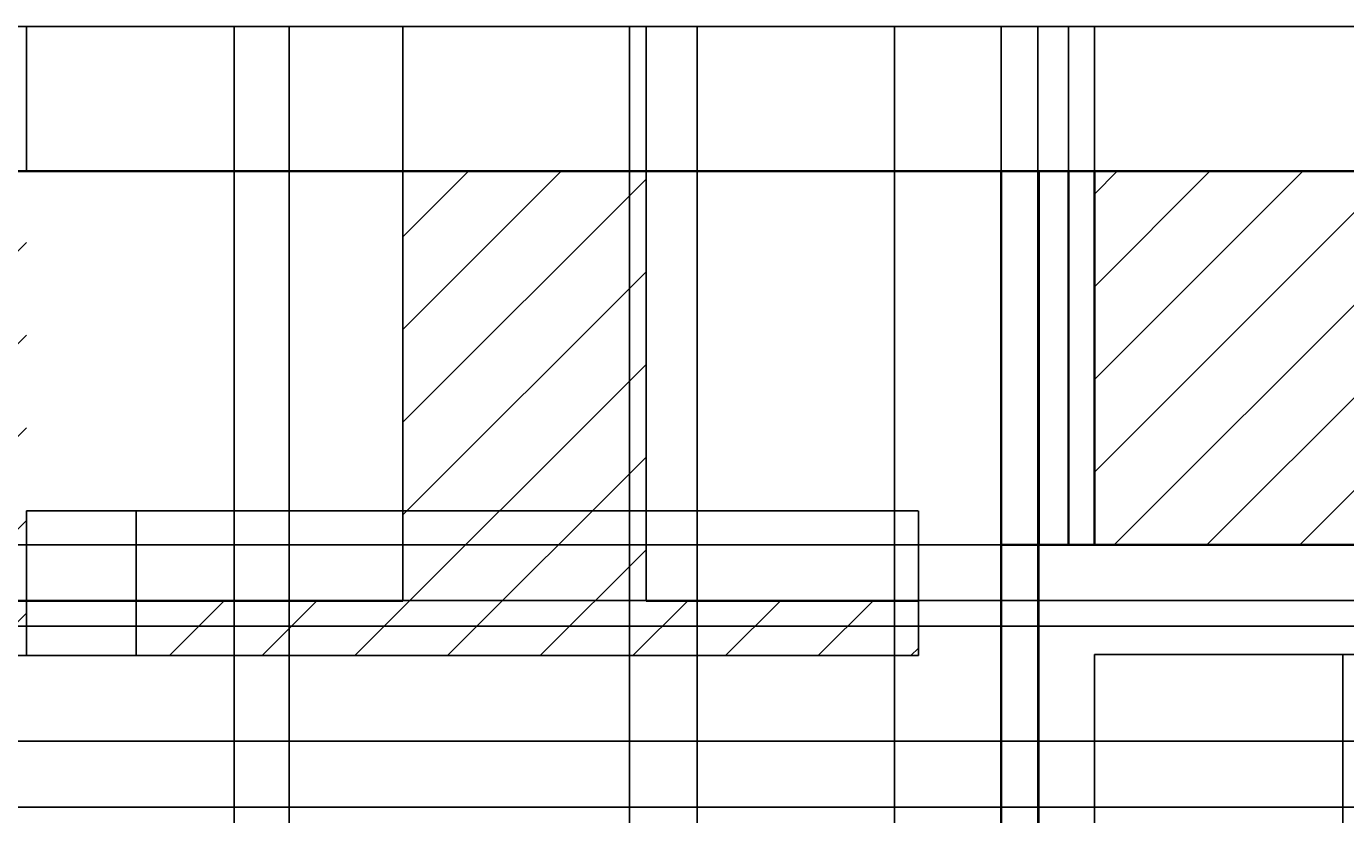
# Model space of a CAD drawing. Units: millimetres. Extents: x 2212 to 7718, y 1114 to 4219.
# Tile 4 of 5: x 4165 to 6466, y 2844 to 4219. Entities that reach past the tile are written whole.
import ezdxf

# ---------------------------------------------------------------- set-up
doc = ezdxf.new("R2010")
doc.units = ezdxf.units.MM
for name, color, linetype, lineweight in [('A-ANNO-DIMS', 2, 'Continuous', 18), ('A-ELEV-PATT', 8, 'Continuous', 13), ('A-EQPM', 4, 'Continuous', 25), ('A-FURN', 7, 'Continuous', 35)]:
    doc.layers.add(name, color=color, linetype=linetype, lineweight=lineweight)
doc.styles.get("Standard").update_dxf_attribs({"font": 'arial.ttf'})
doc.dimstyles.get("Standard").update_dxf_attribs({"dimtxt": 0.18, "dimasz": 0.18, "dimexe": 0.18, "dimexo": 0.0625, "dimgap": 0.09, "dimtad": 0, "dimtih": 1, "dimtoh": 1, "dimdec": 4, "dimzin": 0, "dimdsep": 46, "dimtxsty": 'Standard', "dimcen": 0.09, "dimadec": 0, "dimazin": 0, "dimtfac": 1, "dimtdec": 4, "dimtofl": 0, "dimtmove": 0, "dimatfit": 3, "dimfxl": 1, "dimtolj": 1, "dimtzin": 0, "dimarcsym": 0})

# ---------------------------------------------------------------- blocks, each defined once
blk = doc.blocks.new('*D3')
at = {"layer": 'A-ANNO-DIMS', "color": 0, "lineweight": -2, "transparency": 16777216}
for p, q in [((3659.3, 3966.2), (3659.3, 4218.9)), ((3659.5, 4218.7), (3911.8, 4218.7)), ((4165, 4218.7), (3912.6, 4218.7)), ((4165.1, 3966.2), (4165.1, 4218.9))]:
    blk.add_line(p, q, dxfattribs=at)
at = {"layer": 'A-ANNO-DIMS', "color": 0, "transparency": 16777216}
for points in [[(3659.5, 4218.7), (3659.5, 4218.7), (3659.3, 4218.7)], [(4165, 4218.7), (4165, 4218.7), (4165.1, 4218.7)]]:
    blk.add_solid(points, dxfattribs=at)
at = {"layer": 'Defpoints', "color": 0, "transparency": 16777216}
for p in [(4165.1, 4218.7), (3659.3, 3966.2), (4165.1, 3966.2)]:
    blk.add_point(p, dxfattribs=at)
at = {"layer": 'A-ANNO-DIMS', "color": 0, "transparency": 16777216, "insert": (3912.2, 4218.7), "char_height": 0.18, "attachment_point": 5}
blk.add_mtext('\\A1;505.8', dxfattribs=at)
blk = doc.blocks.new('*D4')
at = {"layer": 'A-ANNO-DIMS', "color": 0, "lineweight": -2, "transparency": 16777216}
for p, q in [((4165.1, 3966.2), (4165.1, 4218.9)), ((4165.3, 4218.7), (4493, 4218.7)), ((4821.4, 4218.7), (4493.8, 4218.7)), ((4821.6, 3966.2), (4821.6, 4218.9))]:
    blk.add_line(p, q, dxfattribs=at)
at = {"layer": 'A-ANNO-DIMS', "color": 0, "transparency": 16777216}
for points in [[(4165.3, 4218.7), (4165.3, 4218.7), (4165.1, 4218.7)], [(4821.4, 4218.7), (4821.4, 4218.7), (4821.6, 4218.7)]]:
    blk.add_solid(points, dxfattribs=at)
at = {"layer": 'Defpoints', "color": 0, "transparency": 16777216}
for p in [(4821.6, 4218.7), (4165.1, 3966.2), (4821.6, 3966.2)]:
    blk.add_point(p, dxfattribs=at)
at = {"layer": 'A-ANNO-DIMS', "color": 0, "transparency": 16777216, "insert": (4493.4, 4218.7), "char_height": 0.18, "attachment_point": 5}
blk.add_mtext('\\A1;656.4', dxfattribs=at)
blk = doc.blocks.new('*D5')
at = {"layer": 'A-ANNO-DIMS', "color": 0, "lineweight": -2, "transparency": 16777216}
for p, q in [((4821.6, 3966.2), (4821.6, 4218.9)), ((4821.8, 4218.7), (5033.2, 4218.7)), ((5245.6, 4218.7), (5034.1, 4218.7)), ((5245.7, 3966.2), (5245.7, 4218.9))]:
    blk.add_line(p, q, dxfattribs=at)
at = {"layer": 'A-ANNO-DIMS', "color": 0, "transparency": 16777216}
for points in [[(4821.8, 4218.7), (4821.8, 4218.7), (4821.6, 4218.7)], [(5245.6, 4218.7), (5245.6, 4218.7), (5245.7, 4218.7)]]:
    blk.add_solid(points, dxfattribs=at)
at = {"layer": 'Defpoints', "color": 0, "transparency": 16777216}
for p in [(5245.7, 4218.7), (4821.6, 3966.2), (5245.7, 3966.2)]:
    blk.add_point(p, dxfattribs=at)
at = {"layer": 'A-ANNO-DIMS', "color": 0, "transparency": 16777216, "insert": (5033.7, 4218.7), "char_height": 0.18, "attachment_point": 5}
blk.add_mtext('\\A1;424.15', dxfattribs=at)
blk = doc.blocks.new('*D6')
at = {"layer": 'A-ANNO-DIMS', "color": 0, "lineweight": -2, "transparency": 16777216}
for p, q in [((5245.7, 3966.2), (5245.7, 4218.9)), ((5245.9, 4218.7), (5555, 4218.7)), ((5865, 4218.7), (5555.8, 4218.7)), ((5865.1, 3966.2), (5865.1, 4218.9))]:
    blk.add_line(p, q, dxfattribs=at)
at = {"layer": 'A-ANNO-DIMS', "color": 0, "transparency": 16777216}
for points in [[(5245.9, 4218.7), (5245.9, 4218.7), (5245.7, 4218.7)], [(5865, 4218.7), (5865, 4218.7), (5865.1, 4218.7)]]:
    blk.add_solid(points, dxfattribs=at)
at = {"layer": 'Defpoints', "color": 0, "transparency": 16777216}
for p in [(5865.1, 4218.7), (5245.7, 3966.2), (5865.1, 3966.2)]:
    blk.add_point(p, dxfattribs=at)
at = {"layer": 'A-ANNO-DIMS', "color": 0, "transparency": 16777216, "insert": (5555.4, 4218.7), "char_height": 0.18, "attachment_point": 5}
blk.add_mtext('\\A1;619.4', dxfattribs=at)
blk = doc.blocks.new('*D7')
at = {"layer": 'A-ANNO-DIMS', "color": 0, "lineweight": -2, "transparency": 16777216}
for p, q in [((5865.1, 3966.2), (5865.1, 4218.9)), ((5865.3, 4218.7), (6264.9, 4218.7)), ((6665, 4218.7), (6265.4, 4218.7)), ((6665.1, 3966.2), (6665.1, 4218.9))]:
    blk.add_line(p, q, dxfattribs=at)
at = {"layer": 'A-ANNO-DIMS', "color": 0, "transparency": 16777216}
for points in [[(5865.3, 4218.7), (5865.3, 4218.7), (5865.1, 4218.7)], [(6665, 4218.7), (6665, 4218.7), (6665.1, 4218.7)]]:
    blk.add_solid(points, dxfattribs=at)
at = {"layer": 'Defpoints', "color": 0, "transparency": 16777216}
for p in [(6665.1, 4218.7), (5865.1, 3966.2), (6665.1, 3966.2)]:
    blk.add_point(p, dxfattribs=at)
at = {"layer": 'A-ANNO-DIMS', "color": 0, "transparency": 16777216, "insert": (6265.1, 4218.7), "char_height": 0.18, "attachment_point": 5}
blk.add_mtext('\\A1;800', dxfattribs=at)
blk = doc.blocks.new('*D10')
at = {"layer": 'A-ANNO-DIMS', "color": 0, "lineweight": -2, "transparency": 16777216}
for p, q in [((4165.1, 3121.4), (4165.1, 3374)), ((4165.3, 3373.8), (4260.5, 3373.8)), ((4356.5, 3373.8), (4261.4, 3373.8)), ((4356.7, 3121.4), (4356.7, 3374))]:
    blk.add_line(p, q, dxfattribs=at)
at = {"layer": 'A-ANNO-DIMS', "color": 0, "transparency": 16777216}
for points in [[(4165.3, 3373.9), (4165.3, 3373.8), (4165.1, 3373.8)], [(4356.5, 3373.9), (4356.5, 3373.8), (4356.7, 3373.8)]]:
    blk.add_solid(points, dxfattribs=at)
at = {"layer": 'Defpoints', "color": 0, "transparency": 16777216}
for p in [(4356.7, 3373.8), (4165.1, 3121.3), (4356.7, 3121.3)]:
    blk.add_point(p, dxfattribs=at)
at = {"layer": 'A-ANNO-DIMS', "color": 0, "transparency": 16777216, "insert": (4260.9, 3373.8), "char_height": 0.18, "attachment_point": 5}
blk.add_mtext('\\A1;191.58', dxfattribs=at)
blk = doc.blocks.new('*D11')
at = {"layer": 'A-ANNO-DIMS', "color": 0, "lineweight": -2, "transparency": 16777216}
for p, q in [((4356.7, 3121.4), (4356.7, 3374)), ((4356.9, 3373.8), (5038.4, 3373.8)), ((5720.6, 3373.8), (5039.1, 3373.8)), ((5720.8, 3121.4), (5720.8, 3374))]:
    blk.add_line(p, q, dxfattribs=at)
at = {"layer": 'A-ANNO-DIMS', "color": 0, "transparency": 16777216}
for points in [[(4356.9, 3373.9), (4356.9, 3373.8), (4356.7, 3373.8)], [(5720.6, 3373.9), (5720.6, 3373.8), (5720.8, 3373.8)]]:
    blk.add_solid(points, dxfattribs=at)
at = {"layer": 'Defpoints', "color": 0, "transparency": 16777216}
for p in [(5720.8, 3373.8), (4356.7, 3121.3), (5720.8, 3121.3)]:
    blk.add_point(p, dxfattribs=at)
at = {"layer": 'A-ANNO-DIMS', "color": 0, "transparency": 16777216, "insert": (5038.7, 3373.8), "char_height": 0.18, "attachment_point": 5}
blk.add_mtext('\\A1;1364', dxfattribs=at)
blk = doc.blocks.new('*D12')
at = {"layer": 'A-ANNO-DIMS', "color": 0, "lineweight": -2, "transparency": 16777216}
for p, q in [((4356.7, 3216.4), (4104, 3216.4)), ((4104.2, 3216.2), (4104.2, 3169)), ((4104.2, 3121.5), (4104.2, 3168.7)), ((4356.7, 3121.3), (4104, 3121.3))]:
    blk.add_line(p, q, dxfattribs=at)
at = {"layer": 'A-ANNO-DIMS', "color": 0, "transparency": 16777216}
for points in [[(4104.2, 3216.2), (4104.2, 3216.2), (4104.2, 3216.4)], [(4104.2, 3121.5), (4104.2, 3121.5), (4104.2, 3121.3)]]:
    blk.add_solid(points, dxfattribs=at)
at = {"layer": 'Defpoints', "color": 0, "transparency": 16777216}
for p in [(4104.2, 3216.4), (4356.7, 3216.4), (4356.7, 3121.3)]:
    blk.add_point(p, dxfattribs=at)
at = {"layer": 'A-ANNO-DIMS', "color": 0, "transparency": 16777216, "insert": (4104.2, 3168.9), "char_height": 0.18, "attachment_point": 5}
blk.add_mtext('\\A1;95.06', dxfattribs=at)
blk = doc.blocks.new('*D28')
at = {"layer": 'A-ANNO-DIMS', "color": 0, "lineweight": -2, "transparency": 16777216}
for p, q in [((5865.1, 2856.7), (2212.5, 2856.7)), ((2212.6, 2856.6), (2212.6, 2802)), ((2212.6, 2747), (2212.6, 2801.6)), ((5865.1, 2746.8), (2212.5, 2746.8))]:
    blk.add_line(p, q, dxfattribs=at)
at = {"layer": 'A-ANNO-DIMS', "color": 0, "transparency": 16777216}
for points in [[(2212.6, 2856.6), (2212.7, 2856.6), (2212.6, 2856.7)], [(2212.6, 2747), (2212.7, 2747), (2212.6, 2746.8)]]:
    blk.add_solid(points, dxfattribs=at)
at = {"layer": 'Defpoints', "color": 0, "transparency": 16777216}
for p in [(2212.6, 2856.7), (5865.1, 2856.7), (5865.1, 2746.8)]:
    blk.add_point(p, dxfattribs=at)
at = {"layer": 'A-ANNO-DIMS', "color": 0, "transparency": 16777216, "insert": (2212.6, 2801.8), "char_height": 0.18, "attachment_point": 5}
blk.add_mtext('\\A1;109.95', dxfattribs=at)
blk = doc.blocks.new('*D29')
at = {"layer": 'A-ANNO-DIMS', "color": 0, "lineweight": -2, "transparency": 16777216}
for p, q in [((5865.1, 3217.2), (2212.5, 3217.2)), ((2212.6, 3217.1), (2212.6, 3037.2)), ((2212.6, 2856.9), (2212.6, 3036.8)), ((5865.1, 2856.7), (2212.5, 2856.7))]:
    blk.add_line(p, q, dxfattribs=at)
at = {"layer": 'A-ANNO-DIMS', "color": 0, "transparency": 16777216}
for points in [[(2212.6, 3217.1), (2212.7, 3217.1), (2212.6, 3217.2)], [(2212.6, 2856.9), (2212.7, 2856.9), (2212.6, 2856.7)]]:
    blk.add_solid(points, dxfattribs=at)
at = {"layer": 'Defpoints', "color": 0, "transparency": 16777216}
for p in [(2212.6, 3217.2), (5865.1, 3217.2), (5865.1, 2856.7)]:
    blk.add_point(p, dxfattribs=at)
at = {"layer": 'A-ANNO-DIMS', "color": 0, "transparency": 16777216, "insert": (2212.6, 3037), "char_height": 0.18, "attachment_point": 5}
blk.add_mtext('\\A1;360.5', dxfattribs=at)
blk = doc.blocks.new('*D30')
at = {"layer": 'A-ANNO-DIMS', "color": 0, "lineweight": -2, "transparency": 16777216}
for p, q in [((5865.1, 3314.4), (2212.5, 3314.4)), ((2212.6, 3314.2), (2212.6, 3266)), ((2212.6, 3217.4), (2212.6, 3265.6)), ((5865.1, 3217.2), (2212.5, 3217.2))]:
    blk.add_line(p, q, dxfattribs=at)
at = {"layer": 'A-ANNO-DIMS', "color": 0, "transparency": 16777216}
for points in [[(2212.6, 3314.2), (2212.7, 3314.2), (2212.6, 3314.4)], [(2212.6, 3217.4), (2212.7, 3217.4), (2212.6, 3217.2)]]:
    blk.add_solid(points, dxfattribs=at)
at = {"layer": 'Defpoints', "color": 0, "transparency": 16777216}
for p in [(2212.6, 3314.4), (5865.1, 3314.4), (5865.1, 3217.2)]:
    blk.add_point(p, dxfattribs=at)
at = {"layer": 'A-ANNO-DIMS', "color": 0, "transparency": 16777216, "insert": (2212.6, 3265.8), "char_height": 0.18, "attachment_point": 5}
blk.add_mtext('\\A1;97.14', dxfattribs=at)
blk = doc.blocks.new('*D31')
at = {"layer": 'A-ANNO-DIMS', "color": 0, "lineweight": -2, "transparency": 16777216}
for p, q in [((5865.1, 3966.2), (2212.5, 3966.2)), ((2212.6, 3966), (2212.6, 3640.5)), ((2212.6, 3314.6), (2212.6, 3640.1)), ((5865.1, 3314.4), (2212.5, 3314.4))]:
    blk.add_line(p, q, dxfattribs=at)
at = {"layer": 'A-ANNO-DIMS', "color": 0, "transparency": 16777216}
for points in [[(2212.6, 3966), (2212.7, 3966), (2212.6, 3966.2)], [(2212.6, 3314.6), (2212.7, 3314.6), (2212.6, 3314.4)]]:
    blk.add_solid(points, dxfattribs=at)
at = {"layer": 'Defpoints', "color": 0, "transparency": 16777216}
for p in [(2212.6, 3966.2), (5865.1, 3966.2), (5865.1, 3314.4)]:
    blk.add_point(p, dxfattribs=at)
at = {"layer": 'A-ANNO-DIMS', "color": 0, "transparency": 16777216, "insert": (2212.6, 3640.3), "char_height": 0.18, "attachment_point": 5}
blk.add_mtext('\\A1;651.8', dxfattribs=at)
blk = doc.blocks.new('*D32')
at = {"layer": 'A-ANNO-DIMS', "color": 0, "lineweight": -2, "transparency": 16777216}
for p, q in [((5865.1, 3314.3), (5865.1, 1113.5)), ((5930.5, 3314.3), (5930.5, 1113.5)), ((5865.3, 1113.7), (5897.4, 1113.7)), ((5930.3, 1113.7), (5898.2, 1113.7))]:
    blk.add_line(p, q, dxfattribs=at)
at = {"layer": 'A-ANNO-DIMS', "color": 0, "transparency": 16777216}
for points in [[(5865.3, 1113.7), (5865.3, 1113.7), (5865.1, 1113.7)], [(5930.3, 1113.7), (5930.3, 1113.7), (5930.5, 1113.7)]]:
    blk.add_solid(points, dxfattribs=at)
at = {"layer": 'Defpoints', "color": 0, "transparency": 16777216}
for p in [(5865.1, 3314.4), (5930.5, 3314.4), (5930.5, 1113.7)]:
    blk.add_point(p, dxfattribs=at)
at = {"layer": 'A-ANNO-DIMS', "color": 0, "transparency": 16777216, "insert": (5897.8, 1113.7), "char_height": 0.18, "attachment_point": 5}
blk.add_mtext('\\A1;65.32', dxfattribs=at)
blk = doc.blocks.new('*D33')
at = {"layer": 'A-ANNO-DIMS', "color": 0, "lineweight": -2, "transparency": 16777216}
for p, q in [((5865.1, 3314.4), (5865.1, 4218.9)), ((5865.3, 4218.7), (5923.5, 4218.7)), ((5982.4, 4218.7), (5924.2, 4218.7)), ((5982.5, 3314.4), (5982.5, 4218.9))]:
    blk.add_line(p, q, dxfattribs=at)
at = {"layer": 'A-ANNO-DIMS', "color": 0, "transparency": 16777216}
for points in [[(5865.3, 4218.7), (5865.3, 4218.7), (5865.1, 4218.7)], [(5982.4, 4218.7), (5982.4, 4218.7), (5982.5, 4218.7)]]:
    blk.add_solid(points, dxfattribs=at)
at = {"layer": 'Defpoints', "color": 0, "transparency": 16777216}
for p in [(5982.5, 4218.7), (5865.1, 3314.4), (5982.5, 3314.4)]:
    blk.add_point(p, dxfattribs=at)
at = {"layer": 'A-ANNO-DIMS', "color": 0, "transparency": 16777216, "insert": (5923.8, 4218.7), "char_height": 0.18, "attachment_point": 5}
blk.add_mtext('\\A1;117.4', dxfattribs=at)
blk = doc.blocks.new('*D34')
at = {"layer": 'A-ANNO-DIMS', "color": 0, "lineweight": -2, "transparency": 16777216}
for p, q in [((5982.5, 3314.4), (5982.5, 4218.9)), ((5982.7, 4218.7), (6004.8, 4218.7)), ((6027.6, 4218.7), (6005.6, 4218.7)), ((6027.8, 3314.4), (6027.8, 4218.9))]:
    blk.add_line(p, q, dxfattribs=at)
at = {"layer": 'A-ANNO-DIMS', "color": 0, "transparency": 16777216}
for points in [[(5982.7, 4218.7), (5982.7, 4218.7), (5982.5, 4218.7)], [(6027.6, 4218.7), (6027.6, 4218.7), (6027.8, 4218.7)]]:
    blk.add_solid(points, dxfattribs=at)
at = {"layer": 'Defpoints', "color": 0, "transparency": 16777216}
for p in [(6027.8, 4218.7), (5982.5, 3314.4), (6027.8, 3314.4)]:
    blk.add_point(p, dxfattribs=at)
at = {"layer": 'A-ANNO-DIMS', "color": 0, "transparency": 16777216, "insert": (6005.2, 4218.7), "char_height": 0.18, "attachment_point": 5}
blk.add_mtext('\\A1;45.24', dxfattribs=at)
blk = doc.blocks.new('*D35')
at = {"layer": 'A-ANNO-DIMS', "color": 0, "lineweight": -2, "transparency": 16777216}
for p, q in [((6027.8, 2972.1), (6027.8, 1113.5)), ((6460.8, 2972.1), (6460.8, 1113.5)), ((6028, 1113.7), (6244, 1113.7)), ((6460.6, 1113.7), (6244.6, 1113.7))]:
    blk.add_line(p, q, dxfattribs=at)
at = {"layer": 'A-ANNO-DIMS', "color": 0, "transparency": 16777216}
for points in [[(6028, 1113.7), (6028, 1113.7), (6027.8, 1113.7)], [(6460.6, 1113.7), (6460.6, 1113.7), (6460.8, 1113.7)]]:
    blk.add_solid(points, dxfattribs=at)
at = {"layer": 'Defpoints', "color": 0, "transparency": 16777216}
for p in [(6027.8, 2972.2), (6460.8, 2972.2), (6460.8, 1113.7)]:
    blk.add_point(p, dxfattribs=at)
at = {"layer": 'A-ANNO-DIMS', "color": 0, "transparency": 16777216, "insert": (6244.3, 1113.7), "char_height": 0.18, "attachment_point": 5}
blk.add_mtext('\\A1;433', dxfattribs=at)
blk = doc.blocks.new('*D36')
at = {"layer": 'A-ANNO-DIMS', "color": 0, "lineweight": -2, "transparency": 16777216}
for p, q in [((6460.9, 3122.9), (7717.8, 3122.9)), ((7717.6, 3122.7), (7717.6, 3047.7)), ((7717.6, 2972.4), (7717.6, 3047.3)), ((6460.9, 2972.2), (7717.8, 2972.2))]:
    blk.add_line(p, q, dxfattribs=at)
at = {"layer": 'A-ANNO-DIMS', "color": 0, "transparency": 16777216}
for points in [[(7717.6, 3122.7), (7717.7, 3122.7), (7717.6, 3122.9)], [(7717.6, 2972.4), (7717.7, 2972.4), (7717.6, 2972.2)]]:
    blk.add_solid(points, dxfattribs=at)
at = {"layer": 'Defpoints', "color": 0, "transparency": 16777216}
for p in [(6460.8, 3122.9), (7717.6, 3122.9), (6460.8, 2972.2)]:
    blk.add_point(p, dxfattribs=at)
at = {"layer": 'A-ANNO-DIMS', "color": 0, "transparency": 16777216, "insert": (7717.6, 3047.5), "char_height": 0.18, "attachment_point": 5}
blk.add_mtext('\\A1;150.68', dxfattribs=at)
blk = doc.blocks.new('*D37')
at = {"layer": 'A-ANNO-DIMS', "color": 0, "lineweight": -2, "transparency": 16777216}
for p, q in [((6027.7, 2972.2), (2212.5, 2972.2)), ((2212.6, 2972), (2212.6, 2914.6)), ((2212.6, 2856.9), (2212.6, 2914.3)), ((5930.4, 2856.7), (2212.5, 2856.7))]:
    blk.add_line(p, q, dxfattribs=at)
at = {"layer": 'A-ANNO-DIMS', "color": 0, "transparency": 16777216}
for points in [[(2212.6, 2972), (2212.7, 2972), (2212.6, 2972.2)], [(2212.6, 2856.9), (2212.7, 2856.9), (2212.6, 2856.7)]]:
    blk.add_solid(points, dxfattribs=at)
at = {"layer": 'Defpoints', "color": 0, "transparency": 16777216}
for p in [(2212.6, 2972.2), (6027.8, 2972.2), (5930.5, 2856.7)]:
    blk.add_point(p, dxfattribs=at)
at = {"layer": 'A-ANNO-DIMS', "color": 0, "transparency": 16777216, "insert": (2212.6, 2914.5), "char_height": 0.18, "attachment_point": 5}
blk.add_mtext('\\A1;115.44', dxfattribs=at)
blk = doc.blocks.new('*D42')
at = {"layer": 'A-ANNO-DIMS', "color": 0, "lineweight": -2, "transparency": 16777216}
for p, q in [((6506, 3217.2), (2212.5, 3217.2)), ((2212.6, 3217.1), (2212.6, 3195)), ((2212.6, 3172.6), (2212.6, 3194.6)), ((6530.4, 3172.4), (2212.5, 3172.4))]:
    blk.add_line(p, q, dxfattribs=at)
at = {"layer": 'A-ANNO-DIMS', "color": 0, "transparency": 16777216}
for points in [[(2212.6, 3217.1), (2212.7, 3217.1), (2212.6, 3217.2)], [(2212.6, 3172.6), (2212.7, 3172.6), (2212.6, 3172.4)]]:
    blk.add_solid(points, dxfattribs=at)
at = {"layer": 'Defpoints', "color": 0, "transparency": 16777216}
for p in [(6506.1, 3217.2), (2212.6, 3172.4), (6530.5, 3172.4)]:
    blk.add_point(p, dxfattribs=at)
at = {"layer": 'A-ANNO-DIMS', "color": 0, "transparency": 16777216, "insert": (2212.6, 3194.8), "char_height": 0.18, "attachment_point": 5}
blk.add_mtext('\\A1;44.855', dxfattribs=at)
blk = doc.blocks.new('*D50')
at = {"layer": 'A-ANNO-DIMS', "color": 0, "lineweight": -2, "transparency": 16777216}
for p, q in [((5865.1, 2746.9), (5865.1, 4218.9)), ((5865.3, 4218.7), (5896.7, 4218.7)), ((5928.9, 4218.7), (5897.5, 4218.7)), ((5929, 2684.6), (5929, 4218.9))]:
    blk.add_line(p, q, dxfattribs=at)
at = {"layer": 'A-ANNO-DIMS', "color": 0, "transparency": 16777216}
for points in [[(5865.3, 4218.7), (5865.3, 4218.7), (5865.1, 4218.7)], [(5928.9, 4218.7), (5928.9, 4218.7), (5929, 4218.7)]]:
    blk.add_solid(points, dxfattribs=at)
at = {"layer": 'Defpoints', "color": 0, "transparency": 16777216}
for p in [(5929, 4218.7), (5865.1, 2746.8), (5929, 2684.5)]:
    blk.add_point(p, dxfattribs=at)
at = {"layer": 'A-ANNO-DIMS', "color": 0, "transparency": 16777216, "insert": (5897.1, 4218.7), "char_height": 0.18, "attachment_point": 5}
blk.add_mtext('\\A1;63.91', dxfattribs=at)
blk = doc.blocks.new('*D69')
at = {"layer": 'A-ANNO-DIMS', "color": 0, "lineweight": -2, "transparency": 16777216}
for p, q in [((4623.4, 2414.9), (4623.4, 4218.9)), ((4623.6, 4218.7), (5150.6, 4218.7)), ((5678.7, 4218.7), (5151.6, 4218.7)), ((5678.9, 2414.9), (5678.9, 4218.9))]:
    blk.add_line(p, q, dxfattribs=at)
at = {"layer": 'A-ANNO-DIMS', "color": 0, "transparency": 16777216}
for points in [[(4623.6, 4218.7), (4623.6, 4218.7), (4623.4, 4218.7)], [(5678.7, 4218.7), (5678.7, 4218.7), (5678.9, 4218.7)]]:
    blk.add_solid(points, dxfattribs=at)
at = {"layer": 'Defpoints', "color": 0, "transparency": 16777216}
for p in [(5678.9, 4218.7), (4623.4, 2414.8), (5678.9, 2414.8)]:
    blk.add_point(p, dxfattribs=at)
at = {"layer": 'A-ANNO-DIMS', "color": 0, "transparency": 16777216, "insert": (5151.1, 4218.7), "char_height": 0.18, "attachment_point": 5}
blk.add_mtext('\\A1;1055.48', dxfattribs=at)
blk = doc.blocks.new('*D70')
at = {"layer": 'A-ANNO-DIMS', "color": 0, "lineweight": -2, "transparency": 16777216}
for p, q in [((4527.5, 2333.4), (4527.5, 4218.9)), ((4527.7, 4218.7), (4575.1, 4218.7)), ((4623.2, 4218.7), (4575.8, 4218.7)), ((4623.4, 2414.9), (4623.4, 4218.9))]:
    blk.add_line(p, q, dxfattribs=at)
at = {"layer": 'A-ANNO-DIMS', "color": 0, "transparency": 16777216}
for points in [[(4527.7, 4218.7), (4527.7, 4218.7), (4527.5, 4218.7)], [(4623.2, 4218.7), (4623.2, 4218.7), (4623.4, 4218.7)]]:
    blk.add_solid(points, dxfattribs=at)
at = {"layer": 'Defpoints', "color": 0, "transparency": 16777216}
for p in [(4623.4, 4218.7), (4623.4, 2414.8), (4527.5, 2333.4)]:
    blk.add_point(p, dxfattribs=at)
at = {"layer": 'A-ANNO-DIMS', "color": 0, "transparency": 16777216, "insert": (4575.4, 4218.7), "char_height": 0.18, "attachment_point": 5}
blk.add_mtext('\\A1;95.87', dxfattribs=at)
blk = doc.blocks.new('*D72')
at = {"layer": 'A-ANNO-DIMS', "color": 0, "lineweight": -2, "transparency": 16777216}
for p, q in [((5216.8, 2499.3), (5216.8, 4218.9)), ((5217, 4218.7), (5275.6, 4218.7)), ((5335, 4218.7), (5276.5, 4218.7)), ((5335.2, 2499.3), (5335.2, 4218.9))]:
    blk.add_line(p, q, dxfattribs=at)
at = {"layer": 'A-ANNO-DIMS', "color": 0, "transparency": 16777216}
for points in [[(5217, 4218.7), (5217, 4218.7), (5216.8, 4218.7)], [(5335, 4218.7), (5335, 4218.7), (5335.2, 4218.7)]]:
    blk.add_solid(points, dxfattribs=at)
at = {"layer": 'Defpoints', "color": 0, "transparency": 16777216}
for p in [(5335.2, 4218.7), (5216.8, 2499.2), (5335.2, 2499.2)]:
    blk.add_point(p, dxfattribs=at)
at = {"layer": 'A-ANNO-DIMS', "color": 0, "transparency": 16777216, "insert": (5276, 4218.7), "char_height": 0.18, "attachment_point": 5}
blk.add_mtext('\\A1;118.35', dxfattribs=at)
blk = doc.blocks.new('*D74')
at = {"layer": 'A-ANNO-DIMS', "color": 0, "lineweight": -2, "transparency": 16777216}
for p, q in [((5335.2, 2434.9), (5335.2, 4218.9)), ((5335.4, 4218.7), (5599.7, 4218.7)), ((5865, 4218.7), (5600.6, 4218.7)), ((5865.1, 2414.9), (5865.1, 4218.9))]:
    blk.add_line(p, q, dxfattribs=at)
at = {"layer": 'A-ANNO-DIMS', "color": 0, "transparency": 16777216}
for points in [[(5335.4, 4218.7), (5335.4, 4218.7), (5335.2, 4218.7)], [(5865, 4218.7), (5865, 4218.7), (5865.1, 4218.7)]]:
    blk.add_solid(points, dxfattribs=at)
at = {"layer": 'Defpoints', "color": 0, "transparency": 16777216}
for p in [(5865.1, 4218.7), (5335.2, 2434.8), (5865.1, 2414.8)]:
    blk.add_point(p, dxfattribs=at)
at = {"layer": 'A-ANNO-DIMS', "color": 0, "transparency": 16777216, "insert": (5600.2, 4218.7), "char_height": 0.18, "attachment_point": 5}
blk.add_mtext('\\A1;529.94', dxfattribs=at)

msp = doc.modelspace()

# ---------------------------------------------------------------- hatches: boundary and pattern name
at = {"layer": 'A-ELEV-PATT'}
h = msp.add_hatch(dxfattribs=at)
h.set_pattern_fill('ANSI31', color=256, scale=36)
h.paths.add_polyline_path([(3153.454, 3966.1829), (2465.1412, 3966.1829), (2465.1412, 3121.3339), (3153.454, 3121.3339)])
h.paths.add_polyline_path([(3659.2976, 3966.1829), (3153.454, 3966.1829), (3153.454, 3121.3339), (3659.2976, 3121.3339)])
h.paths.add_polyline_path([(4165.1412, 3966.1829), (3659.2976, 3966.1829), (3659.2976, 3121.3339), (4165.1412, 3121.3339)])
h.paths.add_polyline_path([(3365.1412, 2266.3983), (2465.1412, 2266.3983), (2465.1412, 1366.1829), (3365.1412, 1366.1829)])
h.paths.add_polyline_path([(4165.1412, 2266.3983), (3365.1412, 2266.3983), (3365.1412, 1366.1829), (4165.1412, 1366.1829)])
h.paths.add_polyline_path([(4965.1412, 2266.3983), (4165.1412, 2266.3983), (4165.1412, 1366.1829), (4965.1412, 1366.1829)])
h.paths.add_polyline_path([(5765.1412, 2266.3983), (4965.1412, 2266.3983), (4965.1412, 1366.1829), (5765.1412, 1366.1829)])
h.paths.add_polyline_path([(6665.1412, 2059.6125), (5865.1412, 2059.6125), (5865.1412, 1366.1829), (6665.1412, 1366.1829)])
h.paths.add_polyline_path([(7465.1412, 2266.3983), (7065.1412, 2266.3983), (7065.1412, 1366.1829), (7465.1412, 1366.1829)])
h.paths.add_polyline_path([(7065.1412, 2266.3983), (6665.1412, 2266.3983), (6665.1412, 1366.1829), (7065.1412, 1366.1829)])
h.paths.add_polyline_path([(7465.1412, 3966.1829), (7065.1412, 3966.1829), (7065.1412, 2266.3983), (7465.1412, 2266.3983)])
h.paths.add_polyline_path([(7065.1412, 3966.1829), (6665.1412, 3966.1829), (6665.1412, 2266.3983), (7065.1412, 2266.3983)])
h.paths.add_polyline_path([(6665.1412, 3966.1829), (6027.7806, 3966.1829), (6027.7806, 3314.3715), (6665.1412, 3314.3715)])
h.paths.add_polyline_path([(5245.7331, 3966.1829), (4821.5849, 3966.1829), (4821.5849, 3216.3983), (4356.7186, 3216.3983), (4356.7186, 3121.3339), (5503.6152, 3121.3339), (5720.779, 3121.3339), (5720.779, 3216.3983), (5245.7331, 3216.3983)])

# ---------------------------------------------------------------- linework, layer by layer
at = {"layer": 'A-EQPM'}
for p, q in [((4821.5849, 3966.1829), (4821.5849, 3216.3983)), ((5245.7331, 3966.1829), (5245.7331, 3216.3983)), ((4821.5849, 3216.3983), (4356.7186, 3216.3983)), ((4356.7186, 3216.3983), (4356.7186, 3121.3339)), ((5245.7331, 3216.3983), (5720.779, 3216.3983)), ((5720.779, 3216.3983), (5720.779, 3121.3339)), ((5865.1412, 3217.2303), (6604.3074, 3217.2303)), ((5930.461, 3217.2303), (5930.461, 2856.7409)), ((4356.7186, 3121.3339), (5503.6152, 3121.3339)), ((5720.779, 3121.3339), (5503.6152, 3121.3339)), ((6027.7806, 3122.866), (6027.7806, 2972.1846)), ((6027.7806, 3122.866), (6460.8234, 3122.866)), ((6460.8234, 3122.866), (6460.8234, 2972.1846)), ((6460.8234, 2972.1846), (6027.7806, 2972.1846)), ((6604.3074, 2856.7409), (5865.1412, 2856.7409))]:
    msp.add_line(p, q, dxfattribs=at)
at = {"layer": 'A-FURN'}
for p, q in [((2465.1412, 3966.1829), (5865.1412, 3966.1829)), ((5865.1412, 3966.1829), (5865.1412, 1366.1829)), ((7465.1412, 3966.1829), (5865.1412, 3966.1829)), ((5930.461, 3966.1829), (5930.461, 3314.3715)), ((5982.5373, 3966.1829), (5982.5373, 3314.3715)), ((6027.7806, 3966.1829), (6027.7806, 3314.3715)), ((5865.1412, 3314.3715), (6665.1412, 3314.3715))]:
    msp.add_line(p, q, dxfattribs=at)

# ---------------------------------------------------------------- dimensions: what is measured, and where the dimension line sits
at = {"layer": 'A-ANNO-DIMS'}
for base, p1, p2, override, picture, middle in [((4165.1412, 4218.6829), (3659.2976, 3966.1829), (4165.1412, 3966.1829), {"dimdec": 1, "dimlfac": 1, "dimrnd": 0, "dimzin": 0, "dimdsep": 46, "dimlunit": 2}, '*D3', (3912.2194, 4218.6829)), ((4821.5849, 4218.6829), (4165.1412, 3966.1829), (4821.5849, 3966.1829), {"dimdec": 1, "dimlfac": 1, "dimrnd": 0, "dimzin": 0, "dimdsep": 46, "dimlunit": 2}, '*D4', (4493.363, 4218.6829)), ((4623.3786, 4218.6829), (4527.5091, 2333.3682), (4623.3786, 2414.8193), {"dimdec": 2, "dimlfac": 1, "dimrnd": 0, "dimzin": 0, "dimdsep": 46, "dimlunit": 2}, '*D70', (4575.4438, 4218.6829)), ((5678.8596, 4218.6829), (4623.3786, 2414.8193), (5678.8596, 2414.8193), {"dimdec": 2, "dimlfac": 1, "dimrnd": 0, "dimzin": 0, "dimdsep": 46, "dimlunit": 2}, '*D69', (5151.1191, 4218.6829)), ((5245.7331, 4218.6829), (4821.5849, 3966.1829), (5245.7331, 3966.1829), {"dimdec": 2, "dimlfac": 1, "dimrnd": 0, "dimzin": 0, "dimdsep": 46, "dimlunit": 2}, '*D5', (5033.659, 4218.6829)), ((5335.1967, 4218.6829), (5216.8434, 2499.2007), (5335.1967, 2499.2007), {"dimdec": 2, "dimlfac": 1, "dimrnd": 0, "dimzin": 0, "dimdsep": 46, "dimlunit": 2}, '*D72', (5276.0201, 4218.6829)), ((5865.1412, 4218.6829), (5245.7331, 3966.1829), (5865.1412, 3966.1829), {"dimdec": 1, "dimlfac": 1, "dimrnd": 0, "dimzin": 0, "dimdsep": 46, "dimlunit": 2}, '*D6', (5555.4371, 4218.6829)), ((5865.1412, 4218.6829), (5335.1967, 2434.8193), (5865.1412, 2414.8193), {"dimdec": 2, "dimlfac": 1, "dimrnd": 0, "dimzin": 0, "dimdsep": 46, "dimlunit": 2}, '*D74', (5600.1689, 4218.6829)), ((6665.1412, 4218.6829), (5865.1412, 3966.1829), (6665.1412, 3966.1829), {"dimdec": 0, "dimlfac": 1, "dimrnd": 0, "dimzin": 0, "dimdsep": 46, "dimlunit": 2}, '*D7', (6265.1412, 4218.6829)), ((5982.5373, 4218.6829), (5865.1412, 3314.3715), (5982.5373, 3314.3715), {"dimdec": 1, "dimlfac": 1, "dimrnd": 0, "dimzin": 0, "dimdsep": 46, "dimlunit": 2}, '*D33', (5923.8392, 4218.6829)), ((5929.0495, 4218.6829), (5865.1412, 2746.7954), (5929.0495, 2684.5306), {"dimdec": 2, "dimlfac": 1, "dimrnd": 0, "dimzin": 0, "dimdsep": 46, "dimlunit": 2}, '*D50', (5897.0953, 4218.6829)), ((6027.7806, 4218.6829), (5982.5373, 3314.3715), (6027.7806, 3314.3715), {"dimdec": 2, "dimlfac": 1, "dimrnd": 0, "dimzin": 0, "dimdsep": 46, "dimlunit": 2}, '*D34', (6005.1589, 4218.6829)), ((4356.7186, 3373.8339), (4165.1412, 3121.3339), (4356.7186, 3121.3339), {"dimdec": 2, "dimlfac": 1, "dimrnd": 0, "dimzin": 0, "dimdsep": 46, "dimlunit": 2}, '*D10', (4260.9299, 3373.8339)), ((5720.779, 3373.8339), (4356.7186, 3121.3339), (5720.779, 3121.3339), {"dimdec": 0, "dimlfac": 1, "dimrnd": 0, "dimzin": 0, "dimdsep": 46, "dimlunit": 2}, '*D11', (5038.7488, 3373.8339)), ((5930.461, 1113.6829), (5865.1412, 3314.3715), (5930.461, 3314.3715), {"dimdec": 2, "dimlfac": 1, "dimrnd": 0, "dimzin": 0, "dimdsep": 46, "dimlunit": 2}, '*D32', (5897.8011, 1113.6829)), ((6460.8234, 1113.6829), (6027.7806, 2972.1846), (6460.8234, 2972.1846), {"dimdec": 0, "dimlfac": 1, "dimrnd": 0, "dimzin": 0, "dimdsep": 46, "dimlunit": 2}, '*D35', (6244.302, 1113.6829))]:
    dim = msp.add_linear_dim(base=base, p1=p1, p2=p2, dimstyle='Standard', override=override, dxfattribs=at)
    dim.commit()
    dim.dimension.update_dxf_attribs({"geometry": picture, "text_midpoint": middle})
for base, p1, p2, override, picture, middle in [((2212.6412, 3966.1829), (5865.1412, 3314.3715), (5865.1412, 3966.1829), {"dimdec": 1, "dimlfac": 1, "dimrnd": 0, "dimzin": 0, "dimdsep": 46, "dimlunit": 2}, '*D31', (2212.6412, 3640.2772)), ((2212.6412, 3314.3715), (5865.1412, 3217.2303), (5865.1412, 3314.3715), {"dimdec": 2, "dimlfac": 1, "dimrnd": 0, "dimzin": 0, "dimdsep": 46, "dimlunit": 2}, '*D30', (2212.6412, 3265.8009)), ((2212.6412, 3172.3755), (6506.0666, 3217.2303), (6530.4592, 3172.3755), {"dimdec": 3, "dimlfac": 1, "dimrnd": 0, "dimzin": 0, "dimdsep": 46, "dimlunit": 2}, '*D42', (2212.6412, 3194.8029)), ((2212.6412, 3217.2303), (5865.1412, 2856.7409), (5865.1412, 3217.2303), {"dimdec": 1, "dimlfac": 1, "dimrnd": 0, "dimzin": 0, "dimdsep": 46, "dimlunit": 2}, '*D29', (2212.6412, 3036.9856)), ((4104.2186, 3216.3983), (4356.7186, 3121.3339), (4356.7186, 3216.3983), {"dimdec": 2, "dimlfac": 1, "dimrnd": 0, "dimzin": 0, "dimdsep": 46, "dimlunit": 2}, '*D12', (4104.2186, 3168.8661)), ((7717.6412, 3122.866), (6460.8234, 2972.1846), (6460.8234, 3122.866), {"dimdec": 2, "dimlfac": 1, "dimrnd": 0, "dimzin": 0, "dimdsep": 46, "dimlunit": 2}, '*D36', (7717.6412, 3047.5253)), ((2212.6412, 2972.1846), (5930.461, 2856.7409), (6027.7806, 2972.1846), {"dimdec": 2, "dimlfac": 1, "dimrnd": 0, "dimzin": 0, "dimdsep": 46, "dimlunit": 2}, '*D37', (2212.6412, 2914.4628)), ((2212.6412, 2856.7409), (5865.1412, 2746.7954), (5865.1412, 2856.7409), {"dimdec": 2, "dimlfac": 1, "dimrnd": 0, "dimzin": 0, "dimdsep": 46, "dimlunit": 2}, '*D28', (2212.6412, 2801.7682))]:
    dim = msp.add_linear_dim(base=base, p1=p1, p2=p2, angle=90, dimstyle='Standard', override=override, dxfattribs=at)
    dim.commit()
    dim.dimension.update_dxf_attribs({"geometry": picture, "text_midpoint": middle})

doc.saveas('drawing.dxf')
